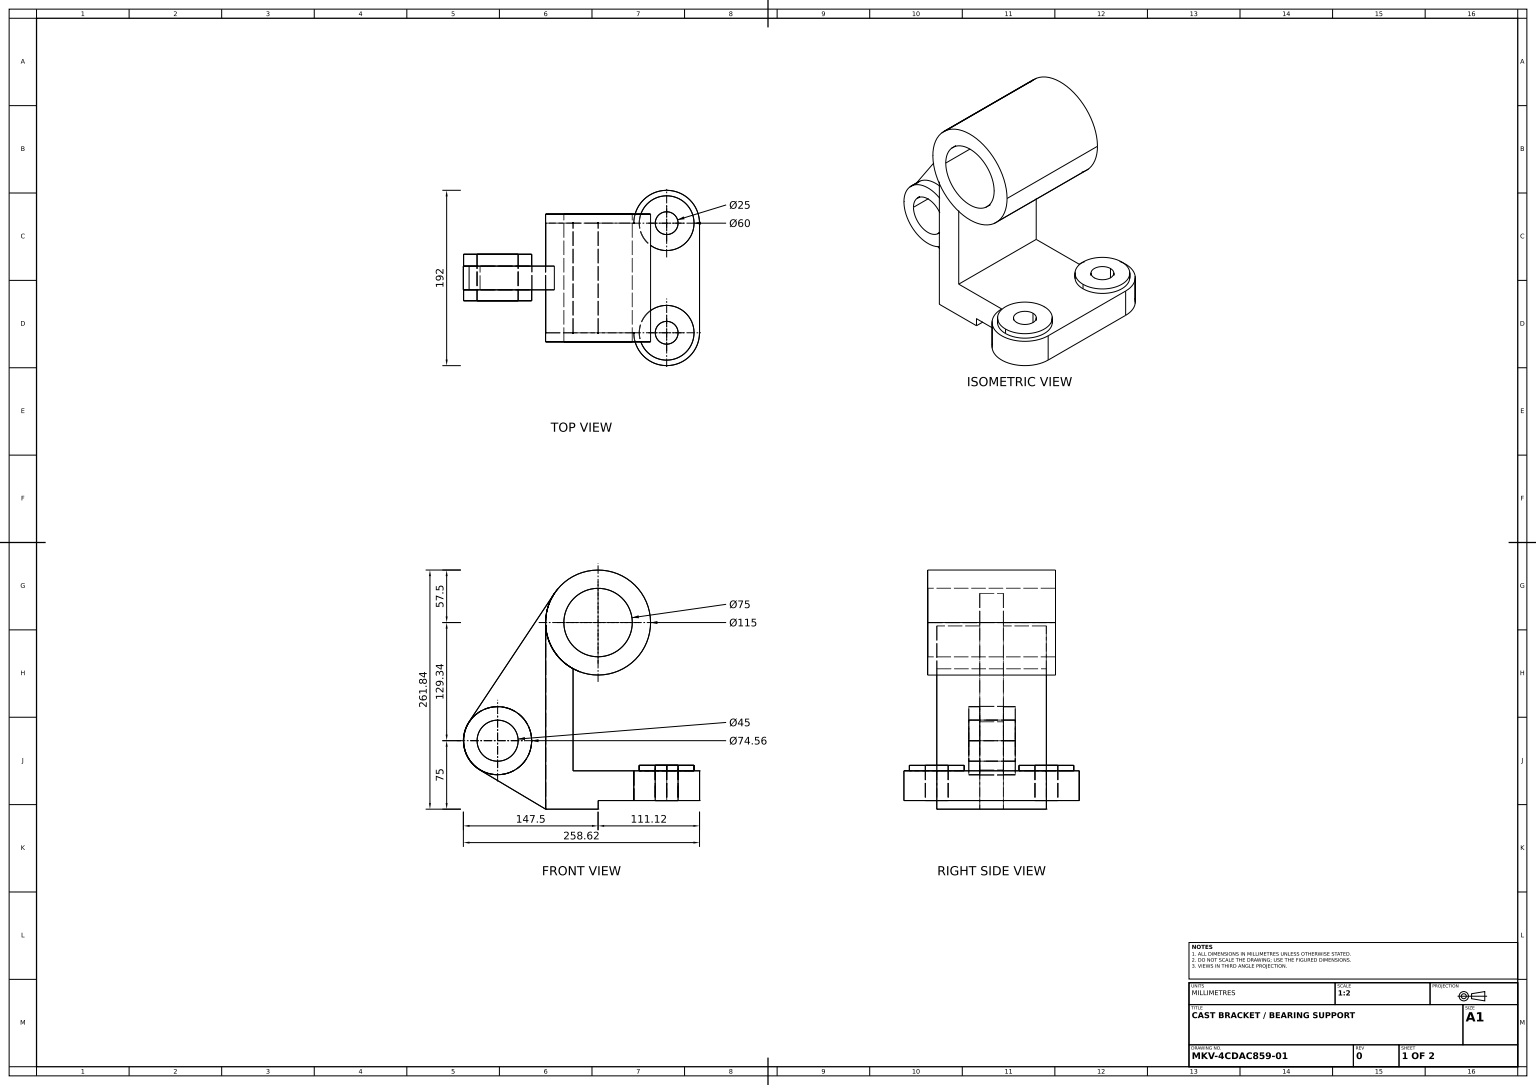
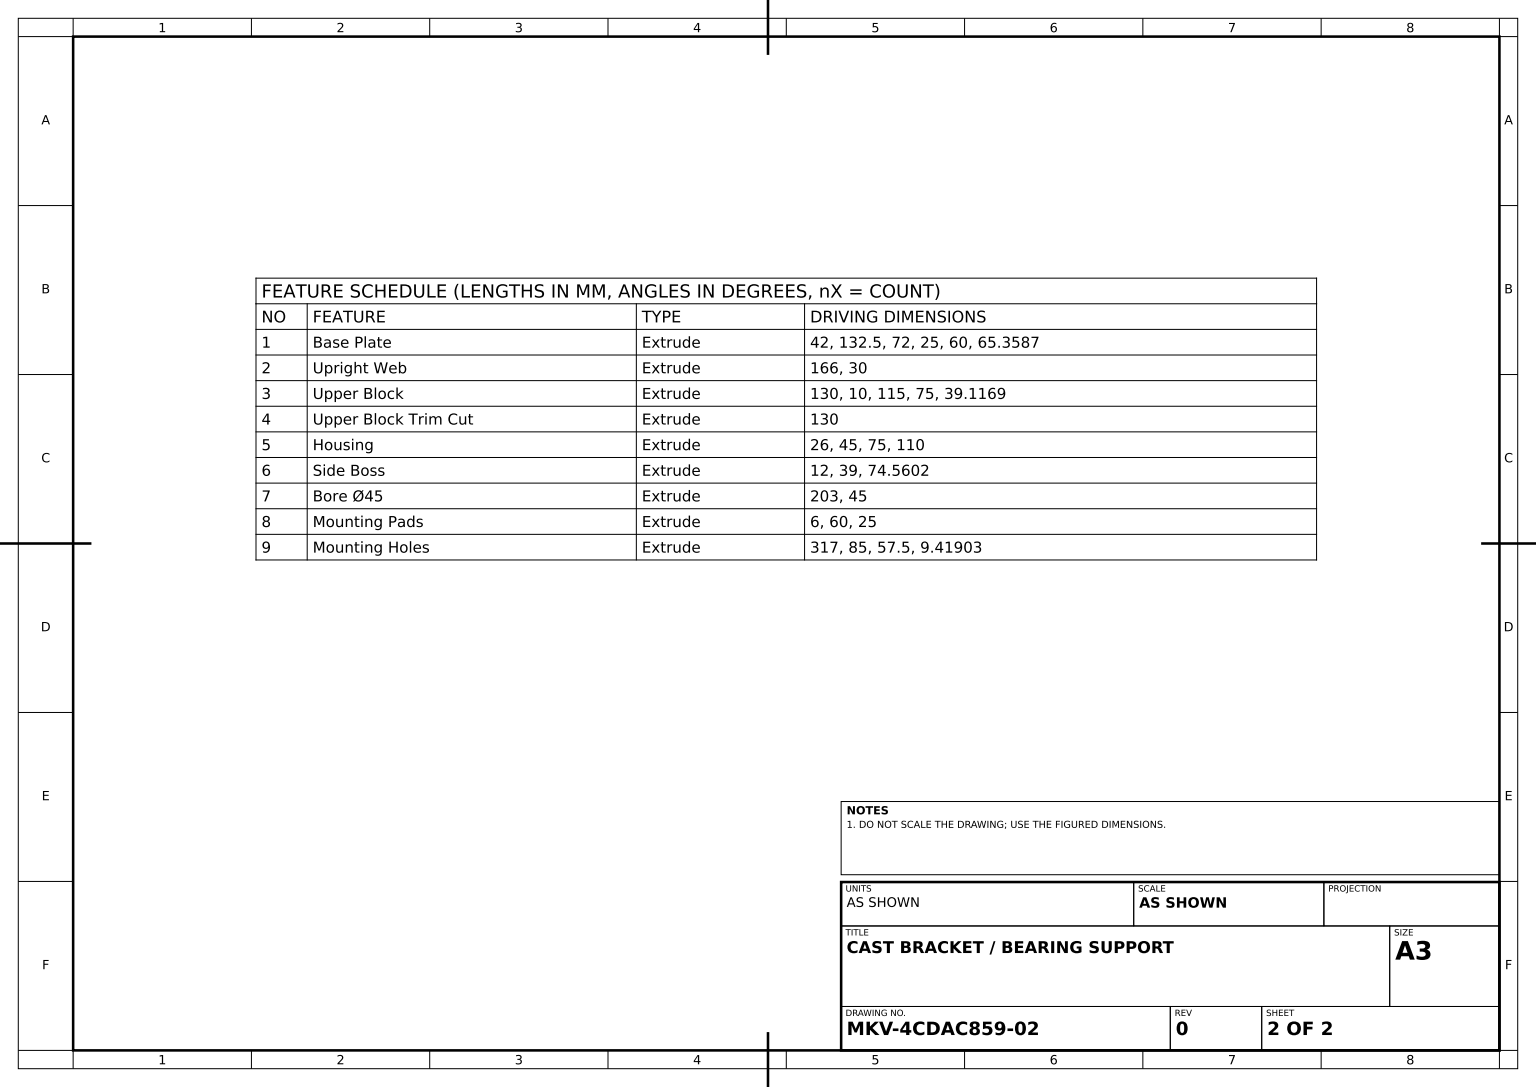
from build123d import *
from build123d.topology import SkipClean

# Parameters (mm, degrees)
BASE_PLATE_PROFILE_R       = 12.5
BASE_PLATE_DEPTH           = 42
UPRIGHT_PROFILE_W          = 30
UPRIGHT_PROFILE_H          = 120
UPRIGHT_WEB_DEPTH          = 166
UPPER_BLOCK_DEPTH          = 10
UPPER_BLOCK_DEPTH_BACK     = 130
UPPER_BLOCK_PROFILE_R      = 57.5
UPPER_BLOCK_PROFILE_R_2    = 37.5
UPPER_BLOCK_TRIM_CUT_DEPTH = 130
HOUSING_PROFILE_R          = 37.5
HOUSING_PROFILE_R_2        = 22.5
HOUSING_DEPTH              = 13
SIDE_BOSS_DEPTH            = 12
SIDE_BOSS_DEPTH_BACK       = 39
SIDE_BOSS_PROFILE_R        = 37.280115622
BORE_45_PROFILE_R          = 22.5
BORE_45_DEPTH              = 203
MOUNTING_PADS_PROFILE_R    = 30
MOUNTING_PADS_PROFILE_R_2  = 12.5
MOUNTING_PADS_DEPTH        = 6
MOUNTING_HOLES_DEPTH       = 85
MOUNTING_HOLES_DEPTH_BACK  = 317
MOUNTING_HOLES_PROFILE_W   = 111
MOUNTING_HOLES_PROFILE_H   = 9.419031608


with BuildPart() as part:
    # Base Plate Profile → Base Plate (new body)
    with BuildSketch(Plane(origin=(0, 0, 0), x_dir=(1, 0, 0), z_dir=(0, 1, 0))):
        with BuildLine():
            Line((-65.358744395, 60), (31.141255605, 60))
            ThreePointArc((31.141255605, 60), (67.141255605, 96), (103.141255605, 60))
            Line((103.141255605, 60), (103.141255605, -60))
            ThreePointArc((103.141255605, -60), (67.141255605, -96), (31.141255605, -60))
            Line((31.141255605, -60), (-65.358744395, -60))
            Line((-65.358744395, -60), (-65.358744395, 60))
        make_face()
        with Locations(Location((67.141255605, -60, 0), (0, 0, 90))):
            Circle(BASE_PLATE_PROFILE_R, mode=Mode.SUBTRACT)
        with Locations(Location((67.141255605, 60, 0), (0, 0, 90))):
            Circle(BASE_PLATE_PROFILE_R, mode=Mode.SUBTRACT)
    extrude(amount=BASE_PLATE_DEPTH)

    # Upright Profile → Upright Web (add)
    with BuildSketch(Plane(origin=(0, 42, 0), x_dir=(1, 0, 0), z_dir=(0, 1, 0))):
        with Locations((-50.358744395, 0)):
            Rectangle(UPRIGHT_PROFILE_W, UPRIGHT_PROFILE_H)
    extrude(amount=UPRIGHT_WEB_DEPTH)

    # Upper Block Profile → Upper Block (add, two sides: drawn at the far end of the back side and taken through both)
    with BuildSketch(Plane.XY.offset(60).offset(-UPPER_BLOCK_DEPTH_BACK)):
        with Locations((-7.975662641, 204.33504045)):
            Circle(UPPER_BLOCK_PROFILE_R)
        with Locations((-7.975662641, 204.33504045)):
            Circle(UPPER_BLOCK_PROFILE_R_2, mode=Mode.SUBTRACT)
    extrude(amount=UPPER_BLOCK_DEPTH + UPPER_BLOCK_DEPTH_BACK)

    # Upper Block Trim Profile → Upper Block Trim Cut (cut)
    with SkipClean():  # the faces are left unmerged after this step: merging them gives an invalid solid
        with BuildSketch(Plane.XY.offset(60)):
            with BuildLine():
                Line((-45.296140552, 208), (-35.358744395, 208))
                Line((-35.358744395, 208), (-35.358744395, 178.714407481))
                ThreePointArc((-35.358744395, 178.714407481), (-43.486916359, 192.285108524), (-45.296140552, 208))
            make_face()
        extrude(amount=-UPPER_BLOCK_TRIM_CUT_DEPTH, mode=Mode.SUBTRACT)

    # Housing Profile → Housing (add, symmetric)
    # profile 1 of 2: a face of its own
    with BuildSketch(Plane.XY):
        with BuildLine():
            ThreePointArc((-80.475662641, 75), (-99.448917842, 42.396170054), (-137.169514756, 42.784382033))
            Line((-137.169514756, 42.784382033), (-65.358744395, 0))
            Line((-65.358744395, 0), (-65.358744395, 200.670080899))
            ThreePointArc((-65.358744395, 200.670080899), (-63.521325311, 219.198733078), (-55.859494126, 236.168806836))
            Line((-55.859494126, 236.168806836), (-149.204248392, 95.761151991))
            ThreePointArc((-149.204248392, 95.761151991), (-107.131815668, 110.897924492), (-80.475662641, 75))
        make_face()
    # profile 2 of 2: a face of its own
    with BuildSketch(Plane.XY):
        with Locations((-117.975662641, 75)):
            Circle(HOUSING_PROFILE_R)
        with Locations(Location((-117.975662641, 75, 0), (0, 0, 180))):
            Circle(HOUSING_PROFILE_R_2, mode=Mode.SUBTRACT)
    extrude(amount=HOUSING_DEPTH, both=True)

    # Side Boss Profile → Side Boss (add, two sides: drawn at the far end of the back side and taken through both)
    with BuildSketch(Plane.XY.offset(13).offset(-SIDE_BOSS_DEPTH_BACK)):
        with Locations((-117.975662641, 75)):
            Circle(SIDE_BOSS_PROFILE_R)
    extrude(amount=SIDE_BOSS_DEPTH + SIDE_BOSS_DEPTH_BACK)

    # Bore Ø45 Profile → Bore Ø45 (cut)
    with BuildSketch(Plane.XY.offset(25)):
        with Locations((-117.975662641, 75)):
            Circle(BORE_45_PROFILE_R)
    extrude(amount=-BORE_45_DEPTH, mode=Mode.SUBTRACT)

    # Mounting Pads Profile → Mounting Pads (add)
    # profile 1 of 2: a face of its own
    with BuildSketch(Plane(origin=(0, 42, 0), x_dir=(1, 0, 0), z_dir=(0, 1, 0))):
        with Locations(Location((67.141255605, -60, 0), (0, 0, 270))):
            Circle(MOUNTING_PADS_PROFILE_R)
        with Locations(Location((67.141255605, -60, 0), (0, 0, 90))):
            Circle(MOUNTING_PADS_PROFILE_R_2, mode=Mode.SUBTRACT)
    # profile 2 of 2: a face of its own
    with BuildSketch(Plane(origin=(0, 42, 0), x_dir=(1, 0, 0), z_dir=(0, 1, 0))):
        with Locations(Location((67.141255605, 60, 0), (0, 0, 270))):
            Circle(MOUNTING_PADS_PROFILE_R)
        with Locations(Location((67.141255605, 60, 0), (0, 0, 90))):
            Circle(MOUNTING_PADS_PROFILE_R_2, mode=Mode.SUBTRACT)
    extrude(amount=MOUNTING_PADS_DEPTH)

    # Mounting Holes Profile → Mounting Holes (cut, two sides: drawn at the far end of the back side and taken through both)
    with BuildSketch(Plane.XY.offset(60).offset(-MOUNTING_HOLES_DEPTH_BACK)):
        with Locations((47.641255605, 4.709515804)):
            Rectangle(MOUNTING_HOLES_PROFILE_W, MOUNTING_HOLES_PROFILE_H)
    extrude(amount=MOUNTING_HOLES_DEPTH + MOUNTING_HOLES_DEPTH_BACK, mode=Mode.SUBTRACT)


solid = part.part
